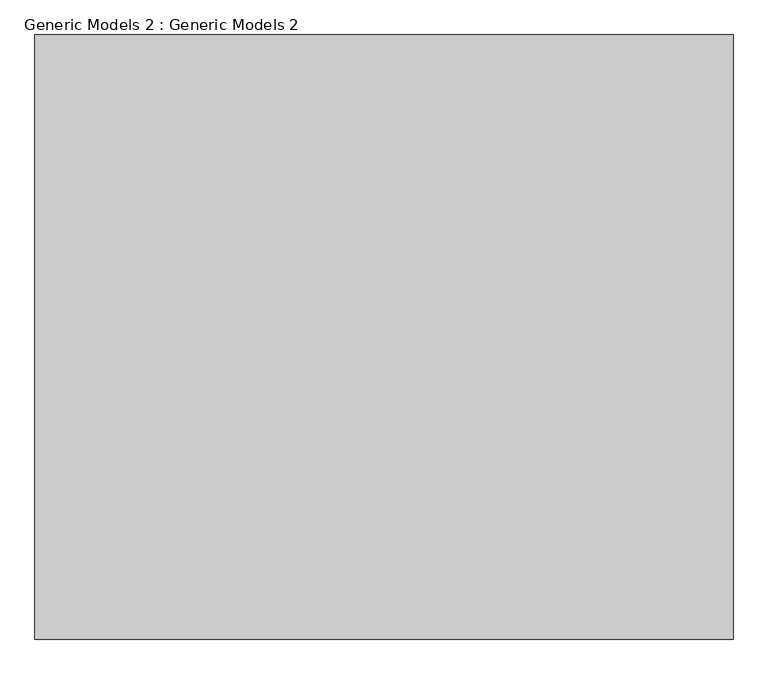
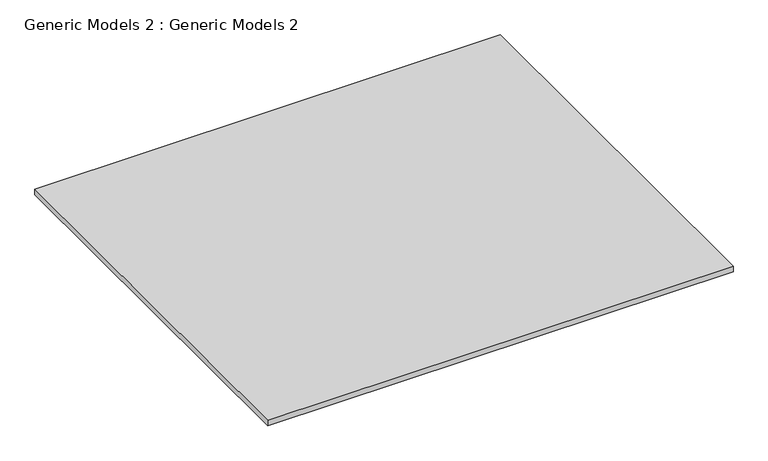
"""IFC4 building model written with IfcOpenShell, lengths in millimetres: proxy geometry, Generic Models 2 : Generic Models 2."""

from ifc_helpers import new_model, si_unit, frame, origin, place, context, project, spatial, polyline, outline, extrude, source, transform, mapped, element, save


def generic_models_2_generic_models_2_479a3e6c(model_context):
    return source(origin(), model_context, "Body", "SweptSolid", [
        extrude(outline(polyline([(-3344.008621, 3894.7560867), (-3344.008621, -16890.5513233), (-27344.2184996, -16890.5513233), (-27344.2184996, 3894.7560867), (-3344.008621, 3894.7560867)])), frame((0.0, 0.0, -304.8), z_axis=(0.0, 0.0, 1.0), x_axis=(1.0, 0.0, 0.0)), (0.0, 0.0, 1.0), 304.8),
    ])


if __name__ == "__main__":
    model = new_model("IFC4")
    model_context = context("Model", 3, world=origin())
    ifc_project = project(units=[si_unit("LENGTHUNIT", "METRE", prefix="MILLI")], contexts=[model_context])
    site = spatial("IfcSite", under=ifc_project)
    building = spatial("IfcBuilding", under=site)
    placement = place(None, origin())
    generic_models_2_generic_models_2_shape = generic_models_2_generic_models_2_479a3e6c(model_context)
    element("IfcBuildingElementProxy", 1, Name="Generic Models 2 : Generic Models 2", ObjectType="Generic Models 2 : Generic Models 2", at=placement, inside=building, context=model_context, shape_type="MappedRepresentation", body=[
        mapped(generic_models_2_generic_models_2_shape, transform((0.0, 0.0, 0.0), x_axis=(1.0, 0.0, 0.0), y_axis=(0.0, 1.0, 0.0), z_axis=(0.0, 0.0, 1.0))),
    ])
    save(model, "model.ifc")
